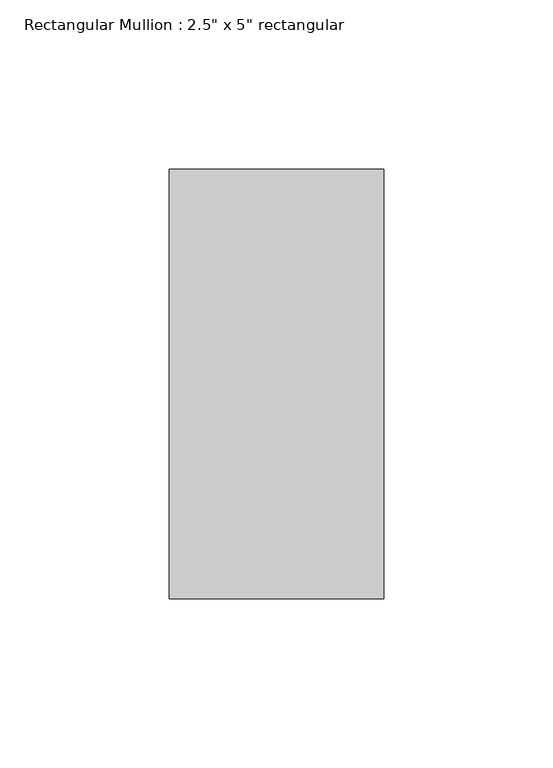
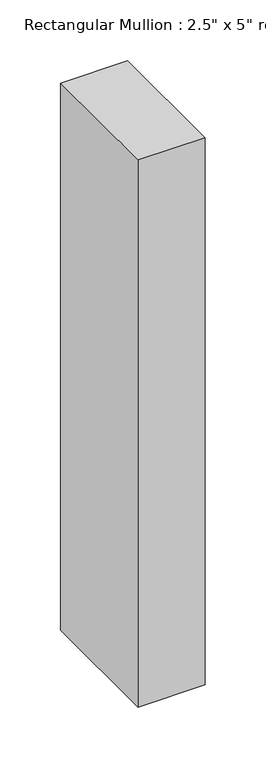
"""IFC4 building model written with IfcOpenShell, lengths in millimetres: member geometry."""

from ifc_helpers import new_model, si_unit, frame, origin, place, context, project, spatial, polyline, outline, extrude, source, transform, mapped, element, save


def member_71656fef(model_context):
    return source(origin(), model_context, "Body", "SweptSolid", [
        extrude(outline(polyline([(0.0, 63.5), (0.0, -63.5), (-63.5, -63.5), (-63.5, 63.5), (0.0, 63.5)])), frame((0.0, 0.0, -548.2166667), z_axis=(0.0, 0.0, 1.0), x_axis=(1.0, 0.0, 0.0)), (0.0, 0.0, 1.0), 548.2166667),
    ])


if __name__ == "__main__":
    model = new_model("IFC4")
    model_context = context("Model", 3, world=origin())
    ifc_project = project(units=[si_unit("LENGTHUNIT", "METRE", prefix="MILLI")], contexts=[model_context])
    site = spatial("IfcSite", under=ifc_project)
    building = spatial("IfcBuilding", under=site)
    placement = place(None, origin())
    member_shape = member_71656fef(model_context)
    element("IfcMember", 1, ObjectType="Rectangular Mullion : 2.5\" x 5\" rectangular", at=placement, inside=building, context=model_context, shape_type="MappedRepresentation", body=[
        mapped(member_shape, transform((0.0, 0.0, 0.0), x_axis=(1.0, 0.0, 0.0), y_axis=(0.0, 1.0, 0.0), z_axis=(0.0, 0.0, 1.0))),
    ])
    save(model, "model.ifc")

# Revit data of these elements
# Type "Rectangular Mullion : 2.5\" x 5\" rectangular"
#   built-in parameter 1007304 = 0.416667 (stored number, unit not read)
#   built-in parameter 1007301 = 0.104167 (stored number, unit not read)
#   built-in parameter 1007300 = 0.104167 (stored number, unit not read)
# Element 1 (IfcMember, "Rectangular Mullion : 2.5\" x 5\" rectangular")
#   Materials on its faces: "Aluminum"
# Materials
#   "Aluminum": class "Metal", colour RGB 247 247 247, transparency 0, Description = "Aluminum 6061", Cost = 0
